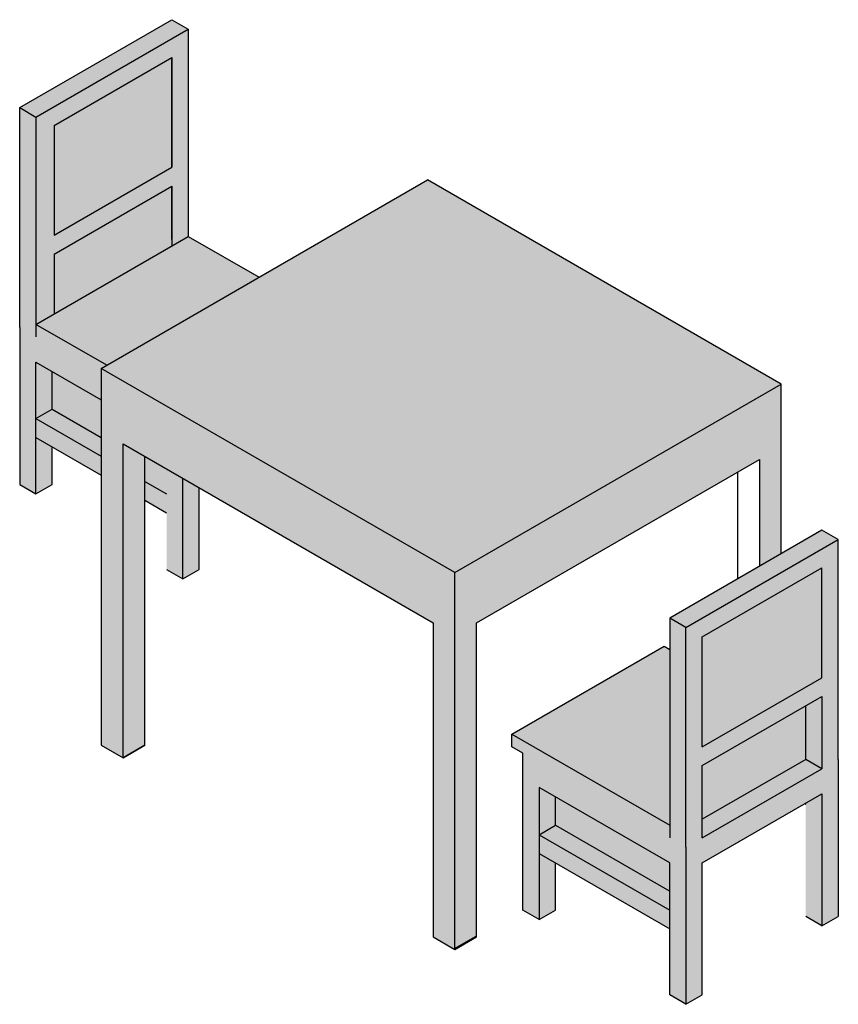
# Model space of a CAD drawing. Units: inches. Extents: x 5998 to 184806, y -27616 to 6737.
# Tile 1 of 3: x 5998 to 7302, y -1227 to 340. Entities that reach past the tile are written whole.
import ezdxf

# ---------------------------------------------------------------- set-up
doc = ezdxf.new("R2010")
doc.units = ezdxf.units.IN
doc.header["$MEASUREMENT"] = 0
doc.layers.add('A-FURN', color=7, linetype='Continuous', lineweight=25)
doc.layers.add('A-FURN-PATT', color=30, linetype='Continuous', lineweight=13)

msp = doc.modelspace()

# ---------------------------------------------------------------- hatches: boundary and pattern name
at = {"layer": 'A-FURN-PATT'}
h = msp.add_hatch(color=256, dxfattribs=at)
h.dxf.hatch_style = 1
h.paths.add_polyline_path([(6266.9, 325.2), (6240.9, 340.2), (5998.5, 200.2), (6024.4, 185.2)])
h.paths.add_polyline_path([(6266.9, 325.2), (6024.4, 185.2), (6024.4, -144.8), (6053.5, -128), (6053.5, -33), (6240.9, 75.2), (6240.9, -9.8), (6240.9, -19.8), (6266.9, -4.8)])
h.paths.add_polyline_path([(6240.9, 280.2), (6240.9, 105.2), (6053.5, -3), (6053.5, 172)], flags=16)
h.paths.add_polyline_path([(6024.4, 185.2), (5998.5, 200.2), (5998.5, -149.8), (5998.5, -399.8), (6024.4, -414.8), (6024.4, -204.8), (6128.4, -264.8), (6128.4, -224.8), (6024.4, -164.8)])
h.paths.add_polyline_path([(6050.4, -219.8), (6024.4, -204.8), (6024.4, -294.8), (6050.4, -279.8)], flags=17)
h.paths.add_polyline_path([(6050.4, -339.8), (6024.4, -324.8), (6024.4, -414.8), (6050.4, -399.8)], flags=17)
h.paths.add_polyline_path([(6024.4, -294.8), (6024.4, -324.8), (6050.4, -339.8), (6128.4, -384.8), (6128.4, -354.8)], flags=17)
h.paths.add_polyline_path([(6050.4, -279.8), (6024.4, -294.8), (6128.4, -354.8), (6128.4, -324.8)], flags=17)
h.paths.add_polyline_path([(6284.2, -404.8), (6258.3, -389.8), (6258.3, -549.8), (6284.2, -534.8)])
h.paths.add_polyline_path([(6258.3, -389.8), (6232.3, -374.8), (6232.3, -534.8), (6258.3, -549.8)])
h.paths.add_polyline_path([(6232.3, -414.8), (6197.6, -394.8), (6197.6, -424.8), (6232.3, -444.8)])
h = msp.add_hatch(color=256, dxfattribs=at)
h.dxf.hatch_style = 1
h.paths.add_polyline_path([(6379.5, -69.8), (6266.9, -4.8), (6024.4, -144.8), (6137, -209.8)])
h.paths.add_polyline_path([(6024.4, -144.8), (6024.4, -164.8), (6128.4, -224.8), (6128.4, -214.8), (6137, -209.8)])
h.paths.add_polyline_path([(6240.9, -19.8), (6240.9, 75.2), (6053.5, -33), (6053.5, -128)])
h.paths.add_polyline_path([(6240.9, 105.2), (6240.9, 280.2), (6053.5, 172), (6053.5, -3)])
h.paths.add_polyline_path([(6128.4, -264.8), (6050.4, -219.8), (6050.4, -279.8), (6128.4, -324.8)])
h.paths.add_polyline_path([(7033.4, -662.3), (7024.7, -657.3), (6782.2, -797.3), (7033.4, -942.3)])
h.paths.add_polyline_path([(6782.2, -797.3), (6782.2, -817.3), (6799.5, -827.3), (7033.4, -962.3), (7033.4, -942.3)])
h.paths.add_polyline_path([(7275.8, -707.3), (7275.8, -532.3), (7085.3, -642.3), (7085.3, -817.3)])
h.paths.add_polyline_path([(7249.9, -837.3), (7249.9, -752.3), (7085.3, -847.3), (7085.3, -932.3)])
h.paths.add_polyline_path([(7275.8, -737.3), (7249.9, -752.3), (7249.9, -837.3), (7275.8, -852.3)])
h.paths.add_polyline_path([(7033.4, -1002.3), (6851.5, -897.3), (6851.5, -942.3), (7033.4, -1047.3)])
h = msp.add_hatch(color=256, dxfattribs=at)
h.dxf.hatch_style = 1
h.paths.add_polyline_path([(7210.9, -239.8), (6648, 85.2), (6128.4, -214.8), (6691.3, -539.8)])
h = msp.add_hatch(color=256, dxfattribs=at)
h.dxf.hatch_style = 1
h.paths.add_polyline_path([(6128.4, -214.8), (6128.4, -814.8), (6163, -834.7), (6163, -834.7), (6163, -334.8), (6656.6, -619.8), (6656.6, -1119.8), (6690.1, -1139.1), (6691.3, -1138.4), (6691.3, -539.8)])
h.paths.add_polyline_path([(6197.6, -354.8), (6163, -334.8), (6163, -834.7), (6197.6, -814.8)], flags=17)
h.paths.add_polyline_path([(6725.9, -619.8), (7176.3, -359.8), (7176.3, -529.8), (7210.9, -509.8), (7210.9, -239.8), (6691.3, -539.8), (6691.3, -1138.4), (6725.9, -1118.4)])
h = msp.add_hatch(color=256, dxfattribs=at)
h.dxf.hatch_style = 1
h.paths.add_polyline_path([(6232.3, -374.8), (6197.6, -354.8), (6197.6, -394.8), (6232.3, -414.8)])
h = msp.add_hatch(color=256, dxfattribs=at)
h.dxf.hatch_style = 1
h.paths.add_polyline_path([(7301.8, -487.3), (7275.8, -472.3), (7033.4, -612.3), (7059.3, -627.3)])
h.paths.add_polyline_path([(7301.8, -487.3), (7059.3, -627.3), (7059.3, -977.3), (7059.3, -1227.3), (7085.3, -1212.3), (7085.3, -1002.3), (7275.8, -892.3), (7275.8, -1102.3), (7301.8, -1087.3), (7301.8, -837.3)])
h.paths.add_polyline_path([(7275.8, -532.3), (7275.8, -707.3), (7085.3, -817.3), (7085.3, -642.3)], flags=16)
h.paths.add_polyline_path([(7275.8, -737.3), (7275.8, -852.3), (7085.3, -962.3), (7085.3, -847.3)], flags=16)
h.paths.add_polyline_path([(7059.3, -627.3), (7033.4, -612.3), (7033.4, -962.3), (6799.5, -827.3), (6799.5, -1077.3), (6825.5, -1092.3), (6825.5, -882.3), (7033.4, -1002.3), (7033.4, -1212.3), (7059.3, -1227.3), (7059.3, -977.3)])
h.paths.add_polyline_path([(6825.5, -957.3), (6825.5, -987.3), (7033.4, -1107.3), (7033.4, -1077.3)], flags=17)
h.paths.add_polyline_path([(6851.5, -942.3), (6825.5, -957.3), (7033.4, -1077.3), (7033.4, -1047.3)], flags=17)
h.paths.add_polyline_path([(6851.5, -1002.3), (6825.5, -987.3), (6825.5, -1092.3), (6851.5, -1077.3)], flags=16)
h.paths.add_polyline_path([(6851.5, -897.3), (6825.5, -882.3), (6825.5, -957.3), (6851.5, -942.3)], flags=17)
h.paths.add_polyline_path([(7275.8, -892.3), (7249.9, -907.3), (7249.9, -1087.3), (7275.8, -1102.3)], flags=17)
h.paths.add_polyline_path([(7249.9, -908.5), (7248.8, -907.9), (7222.8, -922.9), (7249.9, -938.5)], flags=0)
h.paths.add_polyline_path([(7275.8, -852.3), (7249.9, -837.3), (7085.3, -932.3), (7085.3, -962.3)], flags=0)
h = msp.add_hatch(color=256, dxfattribs=at)
h.dxf.hatch_style = 1
h.paths.add_polyline_path([(7275.8, -852.3), (7249.9, -837.3), (7085.3, -932.3), (7085.3, -962.3)])

# ---------------------------------------------------------------- linework, layer by layer
at = {"layer": 'A-FURN'}
for p, q in [((5998.5, 200.2), (6240.9, 340.2)), ((6240.9, 340.2), (6266.9, 325.2)), ((6024.4, 185.2), (6266.9, 325.2)), ((6266.9, 325.2), (6266.9, -4.8)), ((6053.5, 172), (6240.9, 280.2)), ((6240.9, 280.2), (6240.9, 105.2)), ((6240.9, 105.2), (6240.9, 280.2)), ((5998.5, -149.8), (5998.5, 200.2)), ((5998.5, 200.2), (6024.4, 185.2)), ((6024.4, 185.2), (6024.4, -164.8)), ((6053.5, 172), (6053.5, -3)), ((6053.5, -3), (6240.9, 105.2)), ((6128.4, -214.8), (6648, 85.2)), ((7210.9, -239.8), (6648, 85.2)), ((6053.5, -33), (6240.9, 75.2)), ((6240.9, -9.8), (6240.9, 75.2)), ((6240.9, 75.2), (6240.9, -19.8)), ((6024.4, -144.8), (6266.9, -4.8)), ((6266.9, -4.8), (6379.5, -69.8)), ((6053.5, -33), (6053.5, -128)), ((5998.5, -149.8), (5998.5, -399.8)), ((6137, -209.8), (6024.4, -144.8)), ((6024.4, -414.8), (6024.4, -204.8)), ((6024.4, -204.8), (6128.4, -264.8)), ((6691.3, -539.8), (6128.4, -214.8)), ((6128.4, -214.8), (6128.4, -814.8)), ((6050.4, -279.8), (6050.4, -219.8)), ((6691.3, -539.8), (7210.9, -239.8)), ((7210.9, -509.8), (7210.9, -239.8)), ((6024.4, -294.8), (6050.4, -279.8)), ((6050.4, -279.8), (6128.4, -324.8)), ((6024.4, -294.8), (6128.4, -354.8)), ((6024.4, -324.8), (6128.4, -384.8)), ((6050.4, -399.8), (6050.4, -339.8)), ((6163, -834.8), (6163, -334.8)), ((6163, -334.8), (6656.6, -619.8)), ((6197.6, -814.8), (6197.6, -354.8)), ((6725.9, -619.8), (7176.3, -359.8)), ((7176.3, -359.8), (7176.3, -529.8)), ((6258.3, -549.8), (6258.3, -389.8)), ((7141.6, -549.8), (7141.6, -379.8)), ((5998.5, -399.8), (6024.4, -414.8)), ((6024.4, -414.8), (6050.4, -399.8)), ((6197.6, -394.8), (6232.3, -414.8)), ((6284.2, -534.8), (6284.2, -404.8)), ((6197.6, -424.8), (6232.3, -444.8)), ((7275.8, -472.3), (7033.4, -612.3)), ((7301.8, -487.3), (7275.8, -472.3)), ((7059.3, -627.3), (7301.8, -487.3)), ((7301.8, -837.3), (7301.8, -487.3)), ((7085.3, -642.3), (7275.8, -532.3)), ((7275.8, -707.3), (7275.8, -532.3)), ((6232.3, -534.8), (6258.3, -549.8)), ((6258.3, -549.8), (6284.2, -534.8)), ((6691.3, -1139.8), (6691.3, -539.8)), ((6656.6, -619.8), (6656.6, -1119.8)), ((6725.9, -1119.8), (6725.9, -619.8)), ((7059.3, -627.3), (7033.4, -612.3)), ((7033.4, -612.3), (7033.4, -962.3)), ((7059.3, -977.3), (7059.3, -627.3)), ((7085.3, -817.3), (7085.3, -642.3)), ((6782.2, -797.3), (7024.7, -657.3)), ((7024.7, -657.3), (7033.4, -662.3)), ((7085.3, -817.3), (7275.8, -707.3)), ((7085.3, -847.3), (7275.8, -737.3)), ((7249.9, -837.3), (7249.9, -752.3)), ((7275.8, -737.3), (7275.8, -852.3)), ((6782.2, -817.3), (6782.2, -797.3)), ((6782.2, -797.3), (7033.4, -942.3)), ((6128.4, -814.8), (6163, -834.8)), ((6163, -834.8), (6197.6, -814.8)), ((6197.6, -814.8), (6163, -834.7)), ((6799.5, -827.3), (6782.2, -817.3)), ((6799.5, -1077.3), (6799.5, -827.3)), ((7249.9, -837.3), (7085.3, -932.3)), ((7275.8, -852.3), (7249.9, -837.3)), ((7301.8, -837.3), (7301.8, -1087.3)), ((7085.3, -962.3), (7085.3, -847.3)), ((7085.3, -962.3), (7275.8, -852.3)), ((7033.4, -1002.3), (6825.5, -882.3)), ((6825.5, -882.3), (6825.5, -1092.3)), ((7085.3, -1002.3), (7275.8, -892.3)), ((7275.8, -892.3), (7275.8, -1102.3)), ((6851.5, -942.3), (6851.5, -897.3)), ((7248.8, -907.9), (7249.9, -908.5)), ((6825.5, -957.3), (6851.5, -942.3)), ((6851.5, -942.3), (7033.4, -1047.3)), ((6825.5, -957.3), (7033.4, -1077.3)), ((6825.5, -987.3), (7033.4, -1107.3)), ((7059.3, -977.3), (7059.3, -1227.3)), ((6851.5, -1077.3), (6851.5, -1002.3)), ((7033.4, -1212.3), (7033.4, -1002.3)), ((7085.3, -1212.3), (7085.3, -1002.3)), ((6825.5, -1092.3), (6799.5, -1077.3)), ((6825.5, -1092.3), (6851.5, -1077.3)), ((7275.8, -1102.3), (7249.9, -1087.3)), ((7275.8, -1102.3), (7301.8, -1087.3)), ((6656.6, -1119.8), (6691.3, -1139.8)), ((6724.8, -1119.1), (6690.1, -1139.1)), ((6691.3, -1139.8), (6725.9, -1119.8)), ((6725.9, -1119.8), (6724.8, -1119.1)), ((7059.3, -1227.3), (7033.4, -1212.3)), ((7059.3, -1227.3), (7085.3, -1212.3))]:
    msp.add_line(p, q, dxfattribs=at)

doc.saveas('drawing.dxf')
